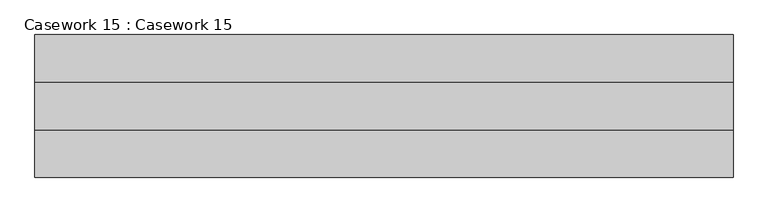
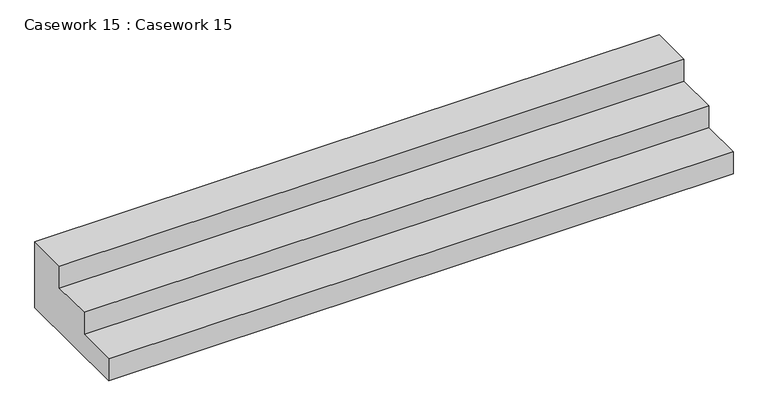
"""IFC4 building model written with IfcOpenShell, lengths in millimetres: furniture geometry, Casework 15 : Casework 15."""

from ifc_helpers import new_model, si_unit, frame, origin, place, context, project, spatial, polyline, outline, extrude, source, transform, mapped, element, save


def casework_15_casework_15_947a4ada(model_context):
    return source(origin(), model_context, "Body", "SweptSolid", [
        extrude(outline(polyline([(4742.2496924, 457.2), (5021.6496924, 457.2), (5021.6496924, 0.0), (4183.4496924, 0.0), (4183.4496924, 152.4), (4462.8496924, 152.4), (4462.8496924, 304.8), (4742.2496924, 304.8), (4742.2496924, 457.2)])), frame((10157.9923267, 0.0, 0.0), z_axis=(1.0, 0.0, 0.0), x_axis=(0.0, 1.0, 0.0)), (0.0, 0.0, 1.0), 4102.1),
    ])


if __name__ == "__main__":
    model = new_model("IFC4")
    model_context = context("Model", 3, world=origin())
    ifc_project = project(units=[si_unit("LENGTHUNIT", "METRE", prefix="MILLI")], contexts=[model_context])
    site = spatial("IfcSite", under=ifc_project)
    building = spatial("IfcBuilding", under=site)
    placement = place(None, origin())
    casework_15_casework_15_shape = casework_15_casework_15_947a4ada(model_context)
    element("IfcFurniture", 1, ObjectType="Casework 15 : Casework 15", at=placement, inside=building, context=model_context, shape_type="MappedRepresentation", body=[
        mapped(casework_15_casework_15_shape, transform((0.0, 0.0, 0.0), x_axis=(1.0, 0.0, 0.0), y_axis=(0.0, 1.0, 0.0), z_axis=(0.0, 0.0, 1.0))),
    ])
    save(model, "model.ifc")
